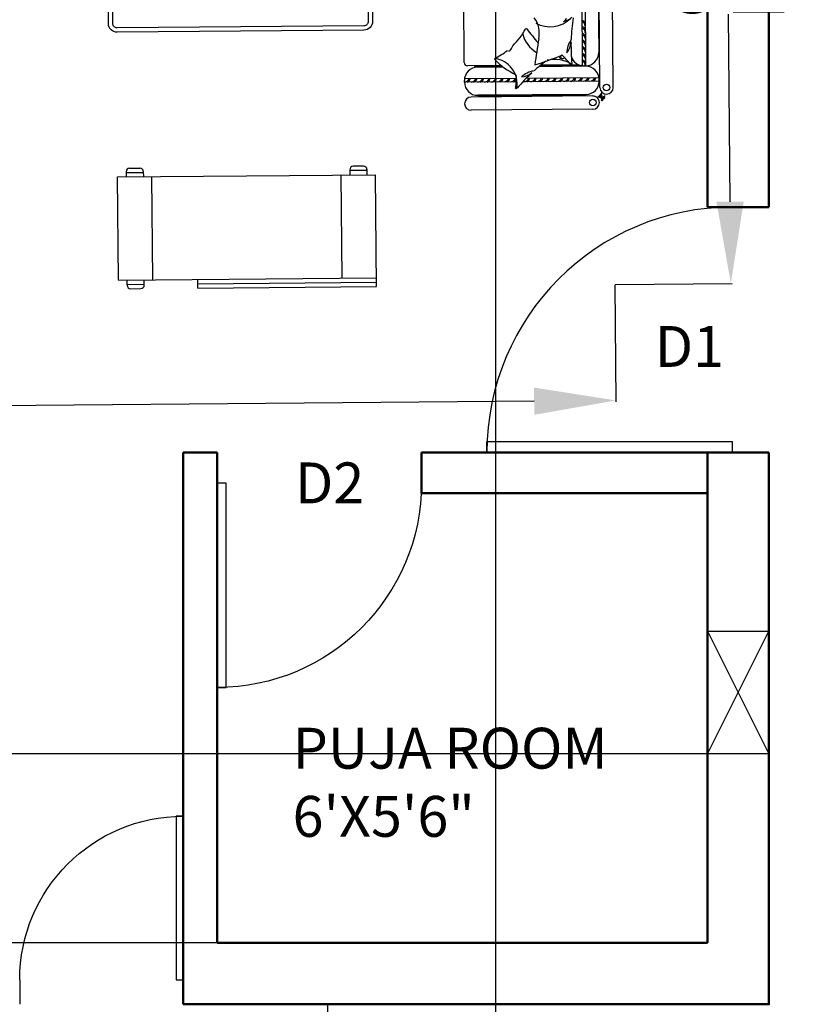
# Model space of a CAD drawing. Units: inches. Extents: x -77 to 516, y -119 to 536.
# Tile 4 of 11: x 264 to 378, y 15 to 159. Entities that reach past the tile are written whole.
import ezdxf

# ---------------------------------------------------------------- set-up
doc = ezdxf.new("R2010")
doc.units = ezdxf.units.IN
doc.header["$MEASUREMENT"] = 0
doc.linetypes.add('ACAD_ISO02W100', pattern=[15, 12, -3])
for name, color, linetype, lineweight in [('A-ANNO-DIMS', 2, 'Continuous', 18), ('A-AREA-IDEN', 170, 'Continuous', 25), ('A-FLOR-PRCH', 40, 'ACAD_ISO02W100', 25), ('doors', 6, 'Continuous', 25), ('furniture', 119, 'Continuous', 18), ('text', 170, 'Continuous', 18), ('walls', 40, 'Continuous', 50), ('windows', 1, 'Continuous', 25)]:
    doc.layers.add(name, color=color, linetype=linetype, lineweight=lineweight)
doc.layers.add('FUR', color=42, linetype='Continuous')
doc.styles.get("Standard").update_dxf_attribs({"font": 'arial.ttf'})
doc.dimstyles.get("Standard").update_dxf_attribs({"dimtxt": 12, "dimasz": 12, "dimexe": 0.18, "dimexo": 0.0625, "dimgap": 0.09, "dimtad": 0, "dimtih": 1, "dimtoh": 1, "dimdec": 1, "dimzin": 0, "dimdsep": 46, "dimlunit": 4, "dimtxsty": 'Standard', "dimcen": 0.09, "dimadec": 0, "dimazin": 0, "dimtfac": 1, "dimtdec": 1, "dimtofl": 0, "dimtmove": 0, "dimatfit": 3, "dimfxl": 1, "dimtolj": 1, "dimtzin": 0, "dimarcsym": 0})

# ---------------------------------------------------------------- blocks, each defined once
blk = doc.blocks.new('*U2')
for p, q in [((0, 0), (0, -6)), ((40, 0), (40, -6))]:
    blk.add_line(p, q)
blk.add_lwpolyline([(0, 0), (0, 40), (1.75, 40), (1.75, 0)], close=True)
blk.add_arc((0, 0), 40, 0, 90)
blk = doc.blocks.new('A$C44A37715')
at = {"layer": 'FUR'}
for p, q in [((2.4248, 3.623), (1.3853, 3.623)), ((1.3853, 3.623), (1.3853, 2.973)), ((2.4248, 3.623), (2.4248, 3.573)), ((2.8153, 3.623), (2.7553, 3.623)), ((2.4248, 3.598), (1.3853, 3.598)), ((2.8853, 3.573), (1.3853, 3.573)), ((1.5853, 3.573), (1.5853, 2.973)), ((2.6853, 3.573), (2.6853, 2.973)), ((2.7353, 3.603), (2.7353, 3.573)), ((2.8353, 3.598), (2.7353, 3.598)), ((2.8353, 3.603), (2.8353, 3.573)), ((2.8853, 3.573), (2.8853, 2.973)), ((2.8853, 2.973), (1.3853, 2.973)), ((1.4353, 2.943), (1.4353, 2.973)), ((1.4353, 2.948), (1.5353, 2.948)), ((1.4553, 2.923), (1.5153, 2.923)), ((1.5353, 2.943), (1.5353, 2.973)), ((2.7353, 2.943), (2.7353, 2.973)), ((2.8353, 2.948), (2.7353, 2.948)), ((2.8153, 2.923), (2.7553, 2.923)), ((2.8353, 2.943), (2.8353, 2.973)), ((0.1193, 2.6037), (0.8259, 2.6037)), ((0.0809, 2.5653), (0.0809, 2.5653)), ((0.1193, 2.5268), (0.8259, 2.5268)), ((0.1577, 2.522), (0.7875, 2.522)), ((0.8644, 2.5653), (0.8644, 2.5653)), ((0, 2.4786), (0, 1.048)), ((0.0384, 2.517), (0.0384, 2.517)), ((0.0768, 2.4786), (0.0768, 1.048)), ((0.1577, 2.5172), (0.7875, 2.5172)), ((0.0809, 2.4404), (0.5248, 2.4404)), ((0.0809, 2.4404), (0.0809, 2.4308)), ((0.0815, 2.4212), (0.5059, 2.4212)), ((0.5619, 2.4212), (0.8638, 2.4212)), ((0.5631, 2.4404), (0.8644, 2.4404)), ((0.8644, 2.4404), (0.8644, 2.4308)), ((0.1577, 2.354), (0.4309, 2.354)), ((0.1591, 2.3508), (0.1687, 2.3508)), ((0.1591, 1.763), (0.1591, 2.3508)), ((0.1783, 1.7636), (0.1783, 2.3502)), ((0.1845, 2.3492), (0.425, 2.3492)), ((0.6381, 2.354), (0.7875, 2.354)), ((0.6442, 2.3492), (0.807, 2.3492)), ((0.1995, 2.3444), (0.4138, 2.3444)), ((0.65, 2.3444), (0.8452, 2.3444)), ((0.8644, 2.3252), (0.8644, 1.7873)), ((0.0822, 1.8399), (0.0822, 2.274)), ((0.2455, 2.204), (0.2455, 2.2321))]:
    blk.add_line(p, q, dxfattribs=at)
for points in [[(2.8805, 2.1325, -0.414214), (2.9305, 2.0825), (2.9305, 1.4325, -0.414214), (2.8805, 1.3825), (1.4454, 1.3825, -0.414214), (1.3954, 1.4325), (1.3954, 2.0825, -0.414214), (1.4454, 2.1325)], [(2.8805, 2.1075, -0.414214), (2.9055, 2.0825), (2.9055, 1.4325, -0.414214), (2.8805, 1.4075), (1.4454, 1.4075, -0.414214), (1.4204, 1.4325), (1.4204, 2.0825, -0.414214), (1.4454, 2.1075)]]:
    blk.add_lwpolyline(points, format="xyb", close=True, dxfattribs=at)
for centre in [(0.1193, 2.5653), (0.0384, 2.4786)]:
    blk.add_circle(centre, 0.0192, dxfattribs=at)
for centre, radius, start, end in [((2.7553, 3.603), 0.02, 90, 180), ((2.8153, 3.603), 0.02, 0, 90), ((1.4553, 2.943), 0.02, 180, 270), ((1.5153, 2.943), 0.02, 270, 0), ((2.7553, 2.943), 0.02, 180, 270), ((2.8153, 2.943), 0.02, 270, 0), ((0.1193, 2.5653), 0.0384, 90, 180), ((0.8259, 2.5653), 0.0384, 0, 90), ((0.0673, 2.5055), 0.0288, 89.3374, 136.5372), ((0.0585, 2.5355), 0.00925, 352.5827, 162.2087), ((0.0466, 2.5342), 0.00508, 309.2756, 53.3144), ((0.0606, 2.5325), 0.00723, 14.0764, 209.9545), ((0.0576, 2.5416), 0.0124, 324.0121, 79.8317), ((0.1577, 2.4404), 0.1152, 123.5982, 144.4891), ((0.0778, 2.5435), 0.0137, 117.9368, 222.4811), ((0.0743, 2.5273), 0.0096, 9.0044, 258.6149), ((0.075, 2.5268), 0.0048, 339.1702, 288.3087), ((0.1193, 2.5653), 0.0384, 180, 270), ((0.8259, 2.5653), 0.0384, 270, 0), ((0.0384, 2.4786), 0.0384, 90, 180), ((0.0384, 2.4786), 0.0384, 0, 90), ((0.1577, 2.4404), 0.0768, 90, 180), ((-0.1974, 3.1303), 0.9988, 312.087, 319.1194), ((0.7075, 2.4517), 0.1492, 169.7702, 262.0088), ((0.5643, 2.4751), 0.0048, 289.2306, 139.1194), ((1.5063, 2.3688), 0.9459, 173.8262, 177.8528), ((0.7875, 2.4404), 0.0768, 0, 90), ((0.1577, 2.4308), 0.0768, 180, 270), ((0.125, 2.4172), 0.0245, 108.4382, 170.6098), ((0.1354, 2.4111), 0.0293, 91.8064, 159.8645), ((0.1635, 2.4172), 0.0245, 108.4382, 170.6098), ((0.1738, 2.4111), 0.0293, 91.8064, 159.8645), ((0.2019, 2.4172), 0.0245, 108.4382, 170.6098), ((0.2122, 2.4111), 0.0293, 91.8064, 159.8645), ((0.2403, 2.4172), 0.0245, 108.4382, 170.6098), ((0.2506, 2.4111), 0.0293, 91.8064, 159.8645), ((0.2787, 2.4172), 0.0245, 108.4382, 170.6098), ((0.289, 2.4111), 0.0293, 91.8064, 159.8645), ((0.3171, 2.4172), 0.0245, 108.4382, 170.6098), ((0.3275, 2.4111), 0.0293, 91.8064, 159.8645), ((0.3555, 2.4172), 0.0245, 108.4382, 170.6098), ((0.3659, 2.4111), 0.0293, 91.8064, 159.8645), ((0.394, 2.4172), 0.0245, 108.4382, 170.6098), ((0.4043, 2.4111), 0.0293, 91.8064, 159.8645), ((0.4324, 2.4172), 0.0245, 108.4382, 170.6098), ((0.4427, 2.4111), 0.0293, 91.8064, 159.8645), ((0.4708, 2.4172), 0.0245, 108.4382, 170.6098), ((0.4811, 2.4111), 0.0293, 91.8064, 159.8645), ((0.445, 2.5022), 0.1246, 277.629, 314.042), ((0.5394, 2.3058), 0.1071, 94.1499, 128.973), ((0.5092, 2.4172), 0.0245, 108.4382, 170.6098), ((0.5195, 2.4111), 0.0293, 91.8064, 159.8645), ((0.586, 2.4172), 0.0245, 108.4382, 170.6098), ((0.5964, 2.4111), 0.0293, 91.8064, 159.8645), ((0.6245, 2.4172), 0.0245, 108.4382, 170.6098), ((0.6348, 2.4111), 0.0293, 91.8064, 159.8645), ((0.6629, 2.4172), 0.0245, 108.4382, 170.6098), ((0.6732, 2.4111), 0.0293, 91.8064, 159.8645), ((0.7013, 2.4172), 0.0245, 108.4382, 170.6098), ((0.7116, 2.4111), 0.0293, 91.8064, 159.8645), ((0.7397, 2.4172), 0.0245, 108.4382, 170.6098), ((0.75, 2.4111), 0.0293, 91.8064, 159.8645), ((0.7781, 2.4172), 0.0245, 108.4382, 170.6098), ((0.7885, 2.4111), 0.0293, 91.8064, 159.8645), ((0.7875, 2.4308), 0.0768, 270, 0), ((0.8165, 2.4172), 0.0245, 108.4382, 170.6098), ((0.8269, 2.4111), 0.0293, 91.8064, 159.8645), ((0.8549, 2.4172), 0.0245, 108.4382, 170.6098), ((0.8653, 2.4111), 0.0293, 91.8064, 159.8645), ((0.1591, 2.274), 0.0768, 90, 180), ((0.1884, 2.3517), 0.0293, 181.8064, 249.8645), ((0.1687, 2.274), 0.0768, 18.3026, 90), ((-0.1974, 3.1303), 0.9988, 305.9918, 311.0925), ((0.3869, 2.0322), 0.4082, 42.8849, 64.0715), ((0.1823, 2.3414), 0.0245, 198.4382, 260.6098), ((0.1884, 2.3133), 0.0293, 181.8064, 249.8645), ((0.1823, 2.303), 0.0245, 198.4382, 260.6098), ((0.2435, 2.338), 0.0048, 39.9755, 185.4148), ((-0.7557, 2.2433), 0.9988, 358.3824, 5.4148), ((0.3395, 2.5014), 0.1892, 238.0983, 282.9802), ((0.972, 2.9488), 0.9459, 219.9755, 224.1671), ((1.3249, 2.0569), 1.0743, 167.2794, 167.2982), ((0.2957, 2.2893), 0.0192, 30.8427, 137.338), ((0.2969, 2.2931), 0.0048, 224.1671, 331.1685), ((-0.7438, 2.0569), 1.0743, 12.7112, 13.5018), ((1.0929, 0.2028), 2.2331, 106.6218, 110.7668), ((-8.7066, 3.7239), 9.2643, 350.48254, 351.42475), ((0.8578, 1.9394), 0.4019, 115.4932, 127.485), ((0.6827, 2.3065), 0.0048, 295.4932, 46.5806), ((0.8452, 2.3252), 0.0192, 0, 90), ((0.1884, 2.2749), 0.0293, 181.8064, 249.8645), ((0.1823, 2.2646), 0.0245, 198.4382, 260.6098), ((0.1884, 2.2365), 0.0293, 181.8064, 249.8645), ((0.3495, 2.2063), 0.1071, 140.4453, 175.2684), ((0.1423, 2.2738), 0.1246, 323.9244, 0.3374), ((0.3635, 2.1287), 0.1625, 11.6119, 60.7251), ((0.8578, 1.9394), 0.4019, 133.4344, 150.9798), ((0.7542, 2.1481), 0.1918, 144.3961, 154.2878), ((0.6022, 2.2569), 0.0048, 33.0156, 144.3961), ((0.1823, 2.2261), 0.0245, 198.4382, 260.6098), ((0.1884, 2.1981), 0.0293, 181.8064, 249.8645), ((0.1823, 2.1877), 0.0245, 198.4382, 260.6098), ((-0.7557, 2.2433), 0.9988, 350.147, 357.3879), ((0.2469, 2.1976), 0.0048, 143.9244, 177.3879), ((0.5796, 2.1587), 0.1531, 167.3915, 215.6783), ((-0.2514, 1.6013), 0.9195, 35.4121, 41.8218), ((0.1884, 2.1596), 0.0293, 181.8064, 249.8645), ((0.1823, 2.1493), 0.0245, 198.4382, 260.6098), ((0.1884, 2.1212), 0.0293, 181.8064, 249.8645), ((0.3624, 1.9521), 0.1703, 60.2042, 134.6584), ((0.5021, 2.1367), 0.0048, 212.7456, 330.9798), ((0.1823, 2.1109), 0.0245, 198.4382, 260.6098), ((0.3028, 1.9936), 0.0998, 100.2155, 131.7497), ((0.2981, 2.0629), 0.0317, 114.2109, 161.7015)]:
    blk.add_arc(centre, radius, start, end, dxfattribs=at)
blk = doc.blocks.new('WIN-18IN')
for p, q in [((18, 0), (0, 9)), ((0, 0), (18, 9))]:
    blk.add_line(p, q)
blk.add_lwpolyline([(0, 9), (18, 9), (18, 0), (0, 0)], close=True)
blk = doc.blocks.new('*D30')
at = {"layer": 'A-ANNO-DIMS', "color": 0, "lineweight": -2, "transparency": 16777216}
for p, q in [((351.13, 120.17), (351.28, 103.03)), ((237.64, 119.18), (237.79, 102.04)), ((339.28, 103.1), (249.78, 102.32)), ((237.78, 102.22), (225.78, 102.12))]:
    blk.add_line(p, q, dxfattribs=at)
at = {"layer": 'A-ANNO-DIMS', "color": 0, "transparency": 16777216}
for points in [[(249.77, 104.32), (249.8, 100.32), (237.78, 102.22)], [(339.27, 105.1), (339.3, 101.1), (351.28, 103.21)]]:
    blk.add_solid(points, dxfattribs=at)
at = {"layer": 'Defpoints', "color": 0, "transparency": 16777216}
for p in [(351.13, 120.23), (237.64, 119.24), (237.78, 102.22)]:
    blk.add_point(p, dxfattribs=at)
at = {"layer": 'A-ANNO-DIMS', "color": 0, "transparency": 16777216, "insert": (140.3, 102.12), "char_height": 12, "attachment_point": 5}
blk.add_mtext('\\A1;SEATING GROUP 114', dxfattribs=at)
blk = doc.blocks.new('*D31')
at = {"layer": 'A-ANNO-DIMS', "color": 0, "lineweight": -2, "transparency": 16777216}
for p, q in [((350.4, 211.74), (367.54, 211.89)), ((367.47, 199.89), (367.71, 172.35)), ((368.05, 132.38), (367.82, 159.91)), ((351.2, 120.23), (368.34, 120.38))]:
    blk.add_line(p, q, dxfattribs=at)
at = {"layer": 'A-ANNO-DIMS', "color": 0, "transparency": 16777216}
for points in [[(369.47, 199.9), (365.47, 199.87), (367.36, 211.88)], [(370.05, 132.4), (366.05, 132.36), (368.16, 120.38)]]:
    blk.add_solid(points, dxfattribs=at)
at = {"layer": 'Defpoints', "color": 0, "transparency": 16777216}
for p in [(350.34, 211.74), (351.13, 120.23), (368.16, 120.38)]:
    blk.add_point(p, dxfattribs=at)
at = {"layer": 'A-ANNO-DIMS', "color": 0, "transparency": 16777216, "insert": (367.76, 166.13), "char_height": 12, "attachment_point": 5}
blk.add_mtext('\\A1;92', dxfattribs=at)
blk = doc.blocks.new('*D37')
at = {"layer": 'A-ANNO-DIMS', "color": 0, "lineweight": -2, "transparency": 16777216}
for p, q in [((373.81, 494.59), (454.58, 494.59)), ((454.4, 482.59), (454.4, 212.81)), ((454.4, -69.41), (454.4, 200.37)), ((309, -81.41), (454.58, -81.41))]:
    blk.add_line(p, q, dxfattribs=at)
at = {"layer": 'A-ANNO-DIMS', "color": 0, "transparency": 16777216}
for points in [[(452.4, 482.59), (456.4, 482.59), (454.4, 494.59)], [(452.4, -69.41), (456.4, -69.41), (454.4, -81.41)]]:
    blk.add_solid(points, dxfattribs=at)
at = {"layer": 'Defpoints', "color": 0, "transparency": 16777216}
for p in [(373.75, 494.59), (454.4, 494.59), (308.93, -81.41)]:
    blk.add_point(p, dxfattribs=at)
at = {"layer": 'A-ANNO-DIMS', "color": 0, "transparency": 16777216, "insert": (454.4, 206.59), "char_height": 12, "attachment_point": 5}
blk.add_mtext('\\A1;576', dxfattribs=at)
blk = doc.blocks.new('*D41')
at = {"layer": 'A-ANNO-DIMS', "color": 0, "lineweight": -2, "transparency": 16777216}
for p, q in [((229.75, 485.53), (229.75, -111.24)), ((333.59, 485.53), (333.59, -111.24)), ((241.75, -111.06), (257.26, -111.06)), ((321.59, -111.06), (306.08, -111.06))]:
    blk.add_line(p, q, dxfattribs=at)
at = {"layer": 'A-ANNO-DIMS', "color": 0, "transparency": 16777216}
for points in [[(241.75, -109.06), (241.75, -113.06), (229.75, -111.06)], [(321.59, -109.06), (321.59, -113.06), (333.59, -111.06)]]:
    blk.add_solid(points, dxfattribs=at)
at = {"layer": 'Defpoints', "color": 0, "transparency": 16777216}
for p in [(229.75, 485.59), (333.59, 485.59), (333.59, -111.06)]:
    blk.add_point(p, dxfattribs=at)
at = {"layer": 'A-ANNO-DIMS', "color": 0, "transparency": 16777216, "insert": (281.67, -111.06), "char_height": 12, "attachment_point": 5}
blk.add_mtext('\\A1;103.84', dxfattribs=at)
blk = doc.blocks.new('*D45')
at = {"layer": 'A-ANNO-DIMS', "color": 0, "lineweight": -2, "transparency": 16777216}
for p, q in [((-15.9, 51.35), (-15.9, 63.35)), ((-15.9, 63.35), (-3.9, 63.35)), ((364.69, 51.35), (-16.08, 51.35)), ((-15.9, 35.59), (-15.9, 39.35)), ((364.69, 23.59), (-16.08, 23.59))]:
    blk.add_line(p, q, dxfattribs=at)
at = {"layer": 'A-ANNO-DIMS', "color": 0, "transparency": 16777216}
for points in [[(-17.9, 39.35), (-13.9, 39.35), (-15.9, 51.35)], [(-17.9, 35.59), (-13.9, 35.59), (-15.9, 23.59)]]:
    blk.add_solid(points, dxfattribs=at)
at = {"layer": 'Defpoints', "color": 0, "transparency": 16777216}
for p in [(-15.9, 51.35), (364.75, 51.35), (364.75, 23.59)]:
    blk.add_point(p, dxfattribs=at)
at = {"layer": 'A-ANNO-DIMS', "color": 0, "transparency": 16777216, "insert": (16.54, 63.35), "char_height": 12, "attachment_point": 5}
blk.add_mtext('\\A1;27.76', dxfattribs=at)

msp = doc.modelspace()

# ---------------------------------------------------------------- linework, layer by layer
at = {"layer": 'A-FLOR-PRCH'}
msp.add_line((308.9336, 14.5884), (308.9336, -81.4116), dxfattribs=at)
at = {"layer": 'walls'}
for p, q in [((364.7501, 131.5884), (364.7501, 485.5884)), ((364.7501, 131.5884), (373.7501, 131.5884)), ((287.7501, 14.5884), (287.7501, 95.5884)), ((287.7501, 95.5884), (292.7501, 95.5884)), ((292.7501, 23.5884), (292.7501, 95.5884)), ((322.7501, 89.5884), (322.7501, 95.5884)), ((322.7501, 95.5884), (373.7501, 95.5884)), ((364.7501, 23.5884), (364.7501, 95.5884)), ((322.7501, 89.5884), (364.7501, 89.5884)), ((292.7501, 23.5884), (364.7501, 23.5884))]:
    msp.add_line(p, q, dxfattribs=at)
for points in [[(373.7501, 131.5884), (373.7501, 494.5884), (13.7501, 494.5884), (13.7501, 14.5884), (239.7501, 14.5884)], [(287.7501, 14.5884), (373.7501, 14.5884), (373.7501, 95.5884)]]:
    msp.add_lwpolyline(points, dxfattribs=at)

# ---------------------------------------------------------------- block references
at = {"layer": 'doors'}
for p, xscale, yscale, zscale, rotation in [((368.3501, 95.5884), 0.9000000000000026, 0.9000000000000026, 0.9000000000000026, 90.00000000000055), ((292.7501, 91.0884), -0.7500000000000016, 0.7500000000000016, 0.7500000000000016, 180)]:
    msp.add_blockref('*U2', p, dxfattribs=dict(at, xscale=xscale, yscale=yscale, zscale=zscale, rotation=rotation))
at = {"layer": 'doors', "xscale": -0.6000000000000032, "yscale": 0.6000000000000032, "zscale": 0.6000000000000032}
msp.add_blockref('*U2', (287.7501, 18.1884), dxfattribs=at)
at = {"layer": 'furniture', "xscale": 25.25763254760833, "yscale": 25.25763254760833, "zscale": 25.25763254760833, "rotation": 180.4978074292498}
msp.add_blockref('A$C44A37715', (350.3392, 211.7368), dxfattribs=at)
at = {"layer": 'windows', "rotation": 270.0000000000005}
msp.add_blockref('WIN-18IN', (364.7497, 69.3473), dxfattribs=at)

# ---------------------------------------------------------------- texts
at = {"layer": 'A-AREA-IDEN', "insert": (303.8149, 55.1737), "char_height": 6, "attachment_point": 1}
msp.add_mtext_dynamic_manual_height_columns('PUJA ROOM\\P6\'X5\'6"', width=105.041962, gutter_width=1, heights=[0], dxfattribs=at)
at = {"layer": 'text', "char_height": 6, "attachment_point": 1}
for s, insert in [('D1', (356.99, 114.1322)), ('D2', (304.166, 94.1065))]:
    msp.add_mtext_dynamic_manual_height_columns(s, width=105.041962, gutter_width=1, heights=[0], dxfattribs=dict(at, insert=insert))

# ---------------------------------------------------------------- dimensions: what is measured, and where the dimension line sits
at = {"layer": 'A-ANNO-DIMS'}
for base, p1, p2, angle, override, picture, middle in [((454.4001, 494.5884), (308.9336, -81.4116), (373.7501, 494.5884), 90, {"dimdec": 0, "dimlfac": 1, "dimrnd": 0, "dimzin": 0, "dimdsep": 46, "dimlunit": 2}, '*D37', (454.4001, 206.5884)), ((368.159, 120.3789), (350.3392, 211.7368), (351.1342, 120.231), 270.497807, {"dimdec": 0, "dimlfac": 1, "dimrnd": 0, "dimzin": 0, "dimdsep": 46, "dimlunit": 2}, '*D31', (367.7615, 166.1318)), ((-15.8999, 51.3473), (364.7501, 23.5884), (364.7501, 51.3473), 90, {"dimdec": 2, "dimlfac": 1, "dimrnd": 0, "dimzin": 0, "dimdsep": 46, "dimlunit": 2}, '*D45', (16.5352, 63.3473))]:
    dim = msp.add_linear_dim(base=base, p1=p1, p2=p2, angle=angle, dimstyle='Standard', override=override, dxfattribs=at)
    dim.commit()
    dim.dimension.update_dxf_attribs({"geometry": picture, "text_midpoint": middle})
dim = msp.add_linear_dim(base=(333.5885, -111.0616), p1=(229.7501, 485.5884), p2=(333.5885, 485.5884), dimstyle='Standard', override={"dimdec": 2, "dimlfac": 1, "dimrnd": 0, "dimzin": 0, "dimdsep": 46, "dimlunit": 2}, dxfattribs=at)
dim.commit()
dim.dimension.update_dxf_attribs({"geometry": '*D41', "text_midpoint": (281.6693, -111.0616)})
dim = msp.add_linear_dim(base=(237.7836, 102.22), p1=(351.1342, 120.231), p2=(237.6357, 119.2448), angle=180.497807, text='SEATING GROUP <>', dimstyle='Standard', override={"dimdec": 0, "dimlfac": 1, "dimrnd": 0, "dimzin": 0, "dimdsep": 46, "dimlunit": 2}, dxfattribs=at)
dim.commit()
dim.dimension.update_dxf_attribs({"geometry": '*D30', "text_midpoint": (140.3025, 102.1158)})

doc.saveas('drawing.dxf')
